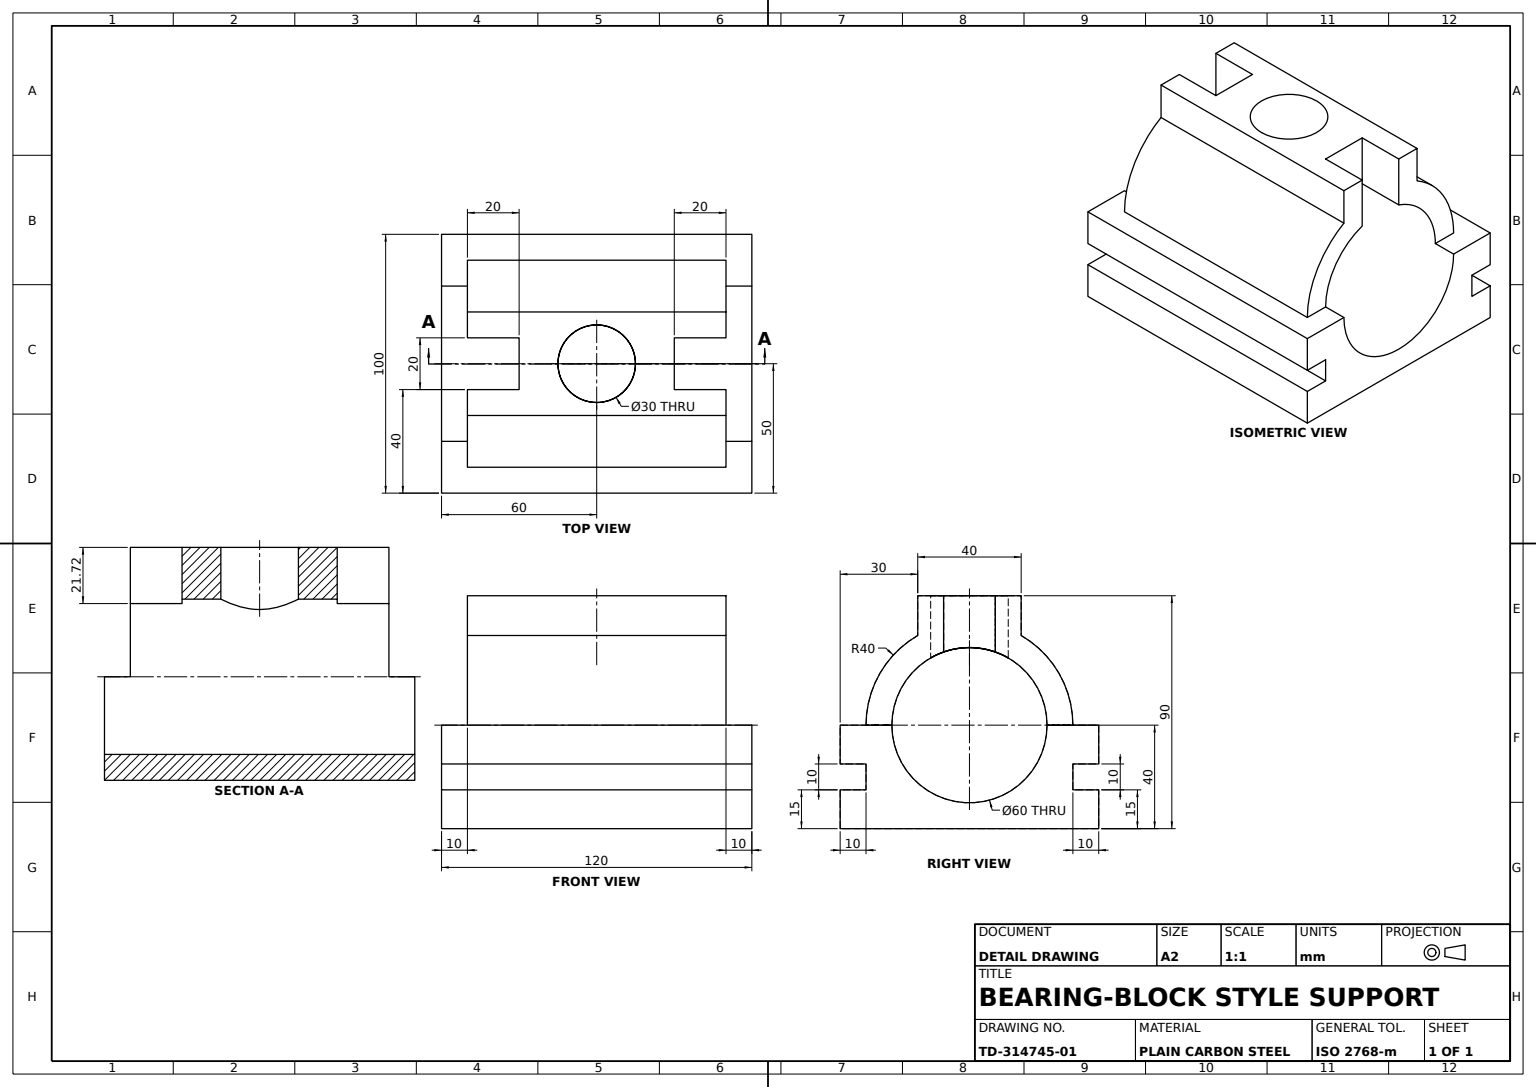
from build123d import *

# Parameters (mm, degrees)
BASE_BLOCK_DEPTH      = 120
BEARING_HOUSING_DEPTH = 100
TOP_SLOTS_SKETCH_W    = 20
TOP_SLOTS_SKETCH_H    = 20
TOP_SLOTS_DEPTH       = 30
TOP_HOLE_SKETCH_R     = 15
TOP_HOLE_30_DEPTH     = 30


with BuildPart() as part:
    # Base Profile Sketch → Base Block (new body)
    with BuildSketch(Plane.XY):
        with BuildLine():
            Line((0, 0), (100, 0))
            Line((100, 0), (100, 15))
            Line((100, 15), (90, 15))
            Line((90, 15), (90, 25))
            Line((90, 25), (100, 25))
            Line((100, 25), (100, 40))
            Line((100, 40), (80, 40))
            ThreePointArc((80, 40), (50, 10), (20, 40))
            Line((20, 40), (0, 40))
            Line((0, 40), (0, 25))
            Line((0, 25), (10, 25))
            Line((10, 25), (10, 15))
            Line((10, 15), (0, 15))
            Line((0, 15), (0, 0))
        make_face()
    extrude(amount=-BASE_BLOCK_DEPTH)

    # Bearing Housing Profile Sketch → Bearing Housing (add)
    with BuildSketch(Plane.XY.offset(-10)):
        with BuildLine():
            ThreePointArc((30, 74.641016151), (15.358983849, 60), (10, 40))
            Line((10, 40), (20, 40))
            ThreePointArc((20, 40), (50, 70), (80, 40))
            Line((80, 40), (90, 40))
            ThreePointArc((90, 40), (84.641016151, 60), (70, 74.641016151))
            ThreePointArc((70, 74.641016151), (50, 80), (30, 74.641016151))
        make_face()
        with BuildLine():
            Line((30, 90), (30, 74.641016151))
            ThreePointArc((30, 74.641016151), (50, 80), (70, 74.641016151))
            Line((70, 74.641016151), (70, 90))
            Line((70, 90), (30, 90))
        make_face()
    extrude(amount=-BEARING_HOUSING_DEPTH)

    # Top Slots Sketch → Top Slots (cut)
    with BuildSketch(Plane(origin=(0, 90, 0), x_dir=(1, 0, 0), z_dir=(0, 1, 0))):
        with Locations((50, 20)):
            Rectangle(TOP_SLOTS_SKETCH_W, TOP_SLOTS_SKETCH_H)
        with Locations((50, 100)):
            Rectangle(TOP_SLOTS_SKETCH_W, TOP_SLOTS_SKETCH_H)
    extrude(amount=-TOP_SLOTS_DEPTH, mode=Mode.SUBTRACT)

    # Top Hole Sketch → Top Hole Ø30 (cut)
    with BuildSketch(Plane(origin=(0, 90, 0), x_dir=(1, 0, 0), z_dir=(0, 1, 0))):
        with Locations(Location((50, 60, 0), (0, 0, 180))):
            Circle(TOP_HOLE_SKETCH_R)
    extrude(amount=-TOP_HOLE_30_DEPTH, mode=Mode.SUBTRACT)


solid = part.part
